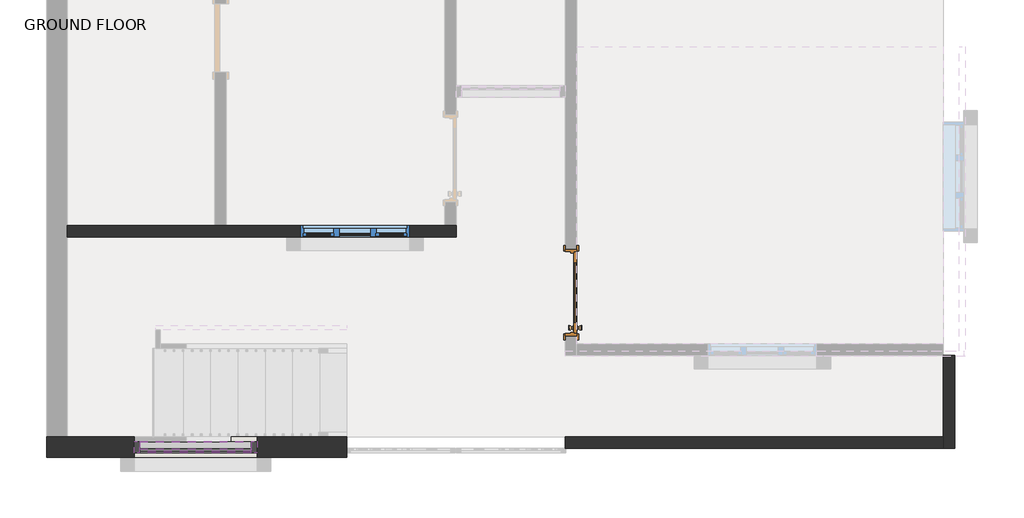
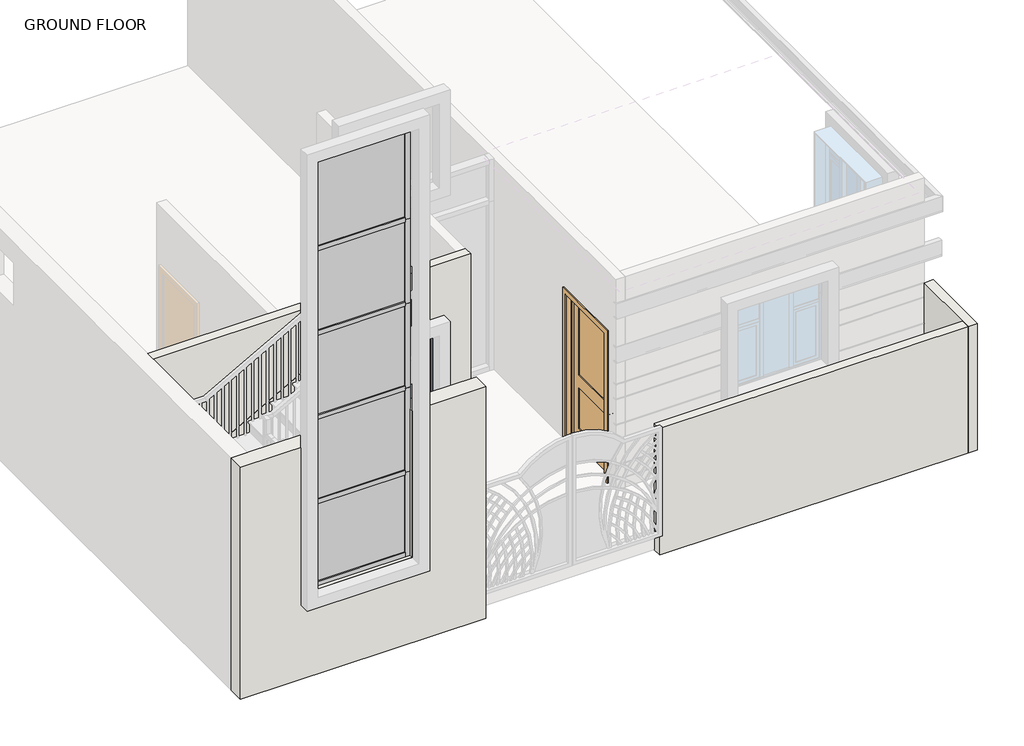
# One storey, part 1 of 7: 16 members, 5 plates, 4 walls, 1 door, 1 window.
"""IFC4 building model written with IfcOpenShell, lengths in millimetres."""

from ifc_helpers import new_model, si_unit, origin, origin_with_axes, place, context, project, spatial, polyline, outline, extrude, faceted_brep, transform, mapped, element, save
from components import door_2e56f206, member_71eb4692, member_a1da5be3, member_0052055d, member_75074519, system_panel_glazed_a6784857, system_panel_glazed_7816ce66, system_panel_glazed_652821f2, window_casement_triple_side_transom_window_4_x_4_9406f89d

model = new_model("IFC4")

# Units and contexts
model_context = context("Model", 3, world=origin())
ifc_project = project(units=[si_unit("LENGTHUNIT", "METRE", prefix="MILLI")], contexts=[model_context])

# Site, building, storey
site = spatial("IfcSite", under=ifc_project)
building = spatial("IfcBuilding", under=site)
storey = spatial("IfcBuildingStorey", under=building, Name="GROUND FLOOR", Elevation=304.8)

# Door
placement = place(None, origin())
door_shape = door_2e56f206(model_context)
element("IfcDoor", 1, ObjectType="Door-Interior-Single-2_Panel-Wood : 36\" x 84\"", at=placement, inside=storey, context=model_context, shape_type="MappedRepresentation", body=[
    mapped(door_shape, transform((-9131.4273867, -1143.8499863, 304.8), x_axis=(0.0, 1.0, 0.0), y_axis=(-1.0, 0.0, 0.0), z_axis=(0.0, 0.0, 1.0))),
])

# Members
member_shape = member_71eb4692(model_context)
element("IfcMember", 2, ObjectType="Rectangular Mullion : 2.5\" x 5\" rectangular", at=placement, inside=storey, context=model_context, shape_type="MappedRepresentation", body=[
    mapped(member_shape, transform((-13947.9023867, -2871.0499863, 7520.3640825), x_axis=(0.0, 0.0, 1.0), y_axis=(0.0, 1.0, 0.0), z_axis=(-1.0, 0.0, 0.0))),
])
element("IfcMember", 3, ObjectType="Rectangular Mullion : 2.5\" x 5\" rectangular", at=placement, inside=storey, context=model_context, shape_type="MappedRepresentation", body=[
    mapped(member_shape, transform((-12703.3023867, -2871.0499863, 1230.3220303), x_axis=(0.0, 0.0, -1.0), y_axis=(0.0, 1.0, 0.0), z_axis=(1.0, 0.0, 0.0))),
])
member_2_shape = member_a1da5be3(model_context)
element("IfcMember", 4, ObjectType="Rectangular Mullion : 2.5\" x 5\" rectangular", at=placement, inside=storey, context=model_context, shape_type="MappedRepresentation", body=[
    mapped(member_2_shape, transform((-13947.9023867, -2871.0499863, 3668.7220303), x_axis=(0.0, 0.0, 1.0), y_axis=(0.0, 1.0, 0.0), z_axis=(-1.0, 0.0, 0.0))),
])
element("IfcMember", 5, ObjectType="Rectangular Mullion : 2.5\" x 5\" rectangular", at=placement, inside=storey, context=model_context, shape_type="MappedRepresentation", body=[
    mapped(member_2_shape, transform((-13947.9023867, -2871.0499863, 6107.1220303), x_axis=(0.0, 0.0, 1.0), y_axis=(0.0, 1.0, 0.0), z_axis=(-1.0, 0.0, 0.0))),
])
element("IfcMember", 6, ObjectType="Rectangular Mullion : 2.5\" x 5\" rectangular", at=placement, inside=storey, context=model_context, shape_type="MappedRepresentation", body=[
    mapped(member_2_shape, transform((-13947.9023867, -2871.0499863, 4887.9220303), x_axis=(0.0, 0.0, 1.0), y_axis=(0.0, 1.0, 0.0), z_axis=(-1.0, 0.0, 0.0))),
])
element("IfcMember", 7, ObjectType="Rectangular Mullion : 2.5\" x 5\" rectangular", at=placement, inside=storey, context=model_context, shape_type="MappedRepresentation", body=[
    mapped(member_2_shape, transform((-13947.9023867, -2871.0499863, 2449.5220303), x_axis=(0.0, 0.0, 1.0), y_axis=(0.0, 1.0, 0.0), z_axis=(-1.0, 0.0, 0.0))),
])
member_3_shape = member_0052055d(model_context)
element("IfcMember", 8, ObjectType="Rectangular Mullion : 2.5\" x 5\" rectangular", at=placement, inside=storey, context=model_context, shape_type="MappedRepresentation", body=[
    mapped(member_3_shape, transform((-12639.8023867, -2871.0499863, 7520.3640825), x_axis=(1.0, 0.0, 0.0), y_axis=(0.0, 1.0, 0.0), z_axis=(0.0, 0.0, 1.0))),
])
element("IfcMember", 9, ObjectType="Rectangular Mullion : 2.5\" x 5\" rectangular", at=placement, inside=storey, context=model_context, shape_type="MappedRepresentation", body=[
    mapped(member_3_shape, transform((-14011.4023867, -2871.0499863, 6107.1220303), x_axis=(-1.0, 0.0, 0.0), y_axis=(0.0, 1.0, 0.0), z_axis=(0.0, 0.0, -1.0))),
])
member_4_shape = member_75074519(model_context)
element("IfcMember", 10, ObjectType="Rectangular Mullion : 2.5\" x 5\" rectangular", at=placement, inside=storey, context=model_context, shape_type="MappedRepresentation", body=[
    mapped(member_4_shape, transform((-14011.4023867, -2871.0499863, 3668.7220303), x_axis=(-1.0, 0.0, 0.0), y_axis=(0.0, 1.0, 0.0), z_axis=(0.0, 0.0, -1.0))),
])
element("IfcMember", 11, ObjectType="Rectangular Mullion : 2.5\" x 5\" rectangular", at=placement, inside=storey, context=model_context, shape_type="MappedRepresentation", body=[
    mapped(member_4_shape, transform((-14011.4023867, -2871.0499863, 4887.9220303), x_axis=(-1.0, 0.0, 0.0), y_axis=(0.0, 1.0, 0.0), z_axis=(0.0, 0.0, -1.0))),
])
element("IfcMember", 12, ObjectType="Rectangular Mullion : 2.5\" x 5\" rectangular", at=placement, inside=storey, context=model_context, shape_type="MappedRepresentation", body=[
    mapped(member_4_shape, transform((-14011.4023867, -2871.0499863, 2449.5220303), x_axis=(-1.0, 0.0, 0.0), y_axis=(0.0, 1.0, 0.0), z_axis=(0.0, 0.0, -1.0))),
])
element("IfcMember", 13, ObjectType="Rectangular Mullion : 2.5\" x 5\" rectangular", at=placement, inside=storey, context=model_context, shape_type="MappedRepresentation", body=[
    mapped(member_4_shape, transform((-12639.8023867, -2871.0499863, 3668.7220303), x_axis=(1.0, 0.0, 0.0), y_axis=(0.0, 1.0, 0.0), z_axis=(0.0, 0.0, 1.0))),
])
element("IfcMember", 14, ObjectType="Rectangular Mullion : 2.5\" x 5\" rectangular", at=placement, inside=storey, context=model_context, shape_type="MappedRepresentation", body=[
    mapped(member_4_shape, transform((-12639.8023867, -2871.0499863, 6107.1220303), x_axis=(1.0, 0.0, 0.0), y_axis=(0.0, 1.0, 0.0), z_axis=(0.0, 0.0, 1.0))),
])
element("IfcMember", 15, ObjectType="Rectangular Mullion : 2.5\" x 5\" rectangular", at=placement, inside=storey, context=model_context, shape_type="MappedRepresentation", body=[
    mapped(member_4_shape, transform((-12639.8023867, -2871.0499863, 4887.9220303), x_axis=(1.0, 0.0, 0.0), y_axis=(0.0, 1.0, 0.0), z_axis=(0.0, 0.0, 1.0))),
])
element("IfcMember", 16, ObjectType="Rectangular Mullion : 2.5\" x 5\" rectangular", at=placement, inside=storey, context=model_context, shape_type="MappedRepresentation", body=[
    mapped(member_4_shape, transform((-14011.4023867, -2871.0499863, 1230.3220303), x_axis=(-1.0, 0.0, 0.0), y_axis=(0.0, 1.0, 0.0), z_axis=(0.0, 0.0, -1.0))),
])
element("IfcMember", 17, ObjectType="Rectangular Mullion : 2.5\" x 5\" rectangular", at=placement, inside=storey, context=model_context, shape_type="MappedRepresentation", body=[
    mapped(member_4_shape, transform((-12639.8023867, -2871.0499863, 2449.5220303), x_axis=(1.0, 0.0, 0.0), y_axis=(0.0, 1.0, 0.0), z_axis=(0.0, 0.0, 1.0))),
])

# Plates
system_panel_glazed_shape = system_panel_glazed_a6784857(model_context)
element("IfcPlate", 18, ObjectType="System Panel : Glazed", at=placement, inside=storey, context=model_context, shape_type="MappedRepresentation", body=[
    mapped(system_panel_glazed_shape, transform((-13325.6023867, -2871.0499863, 6138.8720303), x_axis=(-1.0, 0.0, 0.0), y_axis=(0.0, -1.0, 0.0), z_axis=(0.0, 0.0, 1.0))),
])
system_panel_glazed_2_shape = system_panel_glazed_7816ce66(model_context)
element("IfcPlate", 19, ObjectType="System Panel : Glazed", at=placement, inside=storey, context=model_context, shape_type="MappedRepresentation", body=[
    mapped(system_panel_glazed_2_shape, transform((-13325.6023867, -2871.0499863, 3700.4720303), x_axis=(-1.0, 0.0, 0.0), y_axis=(0.0, -1.0, 0.0), z_axis=(0.0, 0.0, 1.0))),
])
element("IfcPlate", 20, ObjectType="System Panel : Glazed", at=placement, inside=storey, context=model_context, shape_type="MappedRepresentation", body=[
    mapped(system_panel_glazed_2_shape, transform((-13325.6023867, -2871.0499863, 4919.6720303), x_axis=(-1.0, 0.0, 0.0), y_axis=(0.0, -1.0, 0.0), z_axis=(0.0, 0.0, 1.0))),
])
element("IfcPlate", 21, ObjectType="System Panel : Glazed", at=placement, inside=storey, context=model_context, shape_type="MappedRepresentation", body=[
    mapped(system_panel_glazed_2_shape, transform((-13325.6023867, -2871.0499863, 2481.2720303), x_axis=(-1.0, 0.0, 0.0), y_axis=(0.0, -1.0, 0.0), z_axis=(0.0, 0.0, 1.0))),
])
system_panel_glazed_3_shape = system_panel_glazed_652821f2(model_context)
element("IfcPlate", 22, ObjectType="System Panel : Glazed", at=placement, inside=storey, context=model_context, shape_type="MappedRepresentation", body=[
    mapped(system_panel_glazed_3_shape, transform((-13325.6023867, -2871.0499863, 1293.8220303), x_axis=(-1.0, 0.0, 0.0), y_axis=(0.0, -1.0, 0.0), z_axis=(0.0, 0.0, 1.0))),
])

# Walls
element("IfcWall", 23, at=placement, inside=storey, context=model_context, shape_type="Brep", body=[
    faceted_brep([(-11636.5023867, -2756.7499863, 0.0), (-14760.7023867, -2756.7499863, 0.0), (-14989.3023867, -2756.7499863, 0.0), (-14989.3023867, -2756.7499863, 3352.8), (-14760.7023867, -2756.7499863, 3352.8), (-14011.4023867, -2756.7499863, 3352.8), (-14011.4023867, -2756.7499863, 1230.3220303), (-12639.8023867, -2756.7499863, 1230.3220303), (-12639.8023867, -2756.7499863, 3352.8), (-11636.5023867, -2756.7499863, 3352.8), (-14989.3023867, -2985.3499863, 0.0), (-11636.5023867, -2985.3499863, 0.0), (-11636.5023867, -2985.3499863, 3352.8), (-12639.8023867, -2985.3499863, 3352.8), (-12639.8023867, -2985.3499863, 1230.3220303), (-14011.4023867, -2985.3499863, 1230.3220303), (-14011.4023867, -2985.3499863, 3352.8), (-14989.3023867, -2985.3499863, 3352.8)], [[[0, 1, 2, 3, 4, 5, 6, 7, 8, 9]], [[10, 11, 12, 13, 14, 15, 16, 17]], [[2, 1, 0, 11, 10]], [[12, 9, 8, 13]], [[3, 17, 16, 5, 4]], [[0, 9, 12, 11]], [[3, 2, 10, 17]], [[7, 14, 13, 8]], [[15, 6, 5, 16]], [[14, 7, 6, 15]]]),
])
element("IfcWall", 24, ObjectType="INNER WALL 5\"", at=placement, inside=storey, context=model_context, shape_type="Brep", body=[
    faceted_brep([(-14760.7023867, -521.5499863, 304.8), (-10417.3023867, -521.5499863, 304.8), (-10417.3023867, -521.5499863, 3352.8), (-14760.7023867, -521.5499863, 3352.8), (-12157.2023867, -521.5499863, 2438.4), (-10938.0023867, -521.5499863, 2438.4), (-10938.0023867, -521.5499863, 1219.2), (-12157.2023867, -521.5499863, 1219.2), (-14760.7023867, -394.5499863, 304.8), (-14760.7023867, -394.5499863, 3352.8), (-13109.7023867, -394.5499863, 3352.8), (-12982.7023867, -394.5499863, 3352.8), (-10544.3023867, -394.5499863, 3352.8), (-10417.3023867, -394.5499863, 3352.8), (-10417.3023867, -394.5499863, 304.8), (-10544.3023867, -394.5499863, 304.8), (-12982.7023867, -394.5499863, 304.8), (-13109.7023867, -394.5499863, 304.8), (-12157.2023867, -394.5499863, 2438.4), (-12157.2023867, -394.5499863, 1219.2), (-10938.0023867, -394.5499863, 1219.2), (-10938.0023867, -394.5499863, 2438.4)], [[[0, 1, 2, 3], [4, 5, 6, 7]], [[8, 9, 10, 11, 12, 13, 14, 15, 16, 17], [18, 19, 20, 21]], [[1, 0, 8, 17, 16, 15, 14]], [[3, 2, 13, 12, 11, 10, 9]], [[0, 3, 9, 8]], [[2, 1, 14, 13]], [[19, 18, 4, 7]], [[20, 19, 7, 6]], [[21, 20, 6, 5]], [[18, 21, 5, 4]]]),
])
element("IfcWall", 25, ObjectType="INNER WALL 5\"", at=placement, inside=storey, context=model_context, shape_type="Brep", body=[
    faceted_brep([(-4981.7023867, -1842.3499863, 0.0), (-4981.7023867, -2756.7499863, 0.0), (-4981.7023867, -2883.7499863, 0.0), (-4981.7023867, -2883.7499863, 1828.8), (-4981.7023867, -2756.7499863, 1828.8), (-4981.7023867, -1842.3499863, 1828.8), (-4854.7023867, -1842.3499863, 0.0), (-4854.7023867, -1842.3499863, 1828.8), (-4854.7023867, -2883.7499863, 1828.8), (-4854.7023867, -2883.7499863, 0.0)], [[[0, 1, 2, 3, 4, 5]], [[6, 7, 8, 9]], [[2, 1, 0, 6, 9]], [[5, 4, 3, 8, 7]], [[0, 5, 7, 6]], [[3, 2, 9, 8]]]),
])
element("IfcWall", 26, ObjectType="INNER WALL 5\"", at=placement, inside=storey, context=model_context, shape_type="SweptSolid", body=[
    extrude(outline(polyline([(-9198.1023867, -2756.7499863), (-4981.7023867, -2756.7499863), (-4981.7023867, -2883.7499863), (-9198.1023867, -2883.7499863), (-9198.1023867, -2756.7499863)])), origin_with_axes(), (0.0, 0.0, 1.0), 1828.8),
])

# Window
window_casement_triple_side_transom_window_4_x_4_shape = window_casement_triple_side_transom_window_4_x_4_9406f89d(model_context)
element("IfcWindow", 27, ObjectType="Window-Casement-Triple-Side-Transom : window 4' x 4'", at=placement, inside=storey, context=model_context, shape_type="MappedRepresentation", body=[
    mapped(window_casement_triple_side_transom_window_4_x_4_shape, transform((-11547.6023867, -458.0499863, 304.8), x_axis=(-1.0, 0.0, 0.0), y_axis=(0.0, -1.0, 0.0), z_axis=(0.0, 0.0, 1.0))),
])

save(model, "model.ifc")

# Revit data of these elements
# Type "Door-Interior-Single-2_Panel-Wood : 36\" x 84\""
#   Type Mark = "8"
#   Assembly Code = "C1020300"
#   Analytic Construction = "Wooden"
#   Top Rail = 0' - 4 11/16"
#   Thickness = 0' - 1 3/8"
#   Thermal Resistance (R) = 2.5876 (h·ft²·°F)/BTU
#   Swing Angle [instance default] = 90.00°
#   Stiles = 0' - 4 3/4"
#   Rough Width = 3' - 2"
#   Rough Height = 7' - 1"
#   Lock Rail = 0' - 7 1/2"
#   Height = 7' - 0"
#   Width = 3' - 0"
#   Heat Transfer Coefficient (U) = 0.3865 BTU/(h·ft²·°F)
#   Bottom Rail = 0' - 9 1/8"
#   Trim Material = Cherry
#   Panel Material = Cherry
#   Frame Material = Cherry
#   Door Handle Material = Aluminum
#   Visual Light Transmittance = 0
#   Solar Heat Gain Coefficient = 0
#   Wall Closure = (empty or 0)
#   Function = (empty or 0)
# Type "Rectangular Mullion : 2.5\" x 5\" rectangular"
#   built-in parameter 1007304 = 0.416667 (stored number, unit not read)
#   built-in parameter 1007301 = 0.104167 (stored number, unit not read)
#   built-in parameter 1007300 = 0.104167 (stored number, unit not read)
# Type "System Panel : Glazed"
#   Construction Type Id = "GSP4R"
#   Analytic Construction = "1/8 in Pilkington single glazing"
#   Visual Light Transmittance = 0.9
#   Solar Heat Gain Coefficient = 0.86
#   Heat Transfer Coefficient (U) = 1.18115 BTU/(h·ft²·°F)
#   Define Thermal Properties by = 1
# Type
#   Assembly Code = "B2010"
#   Layers, outside or top first: 0' - 9" "OUTER WALL" (function 1)
# Type "INNER WALL 5\""
#   Assembly Code = "B2010"
#   Layers, outside or top first: 0' - 5" "OUTER WALL" (function 1)
# Type "Window-Casement-Triple-Side-Transom : window 4' x 4'"
#   Type Mark = "22"
#   Fire Rating = "0.5h"
#   Assembly Code = "B2020100"
#   Analytic Construction = "Double glazing - domestic"
#   Window Width = 1' - 4"
#   Window Inset [instance default] = 0' - 0 5/8"
#   Wall Thickness [instance default] = 0' - 6"
#   Visual Light Transmittance = 0.81
#   Transom Height Ratio = 0.3
#   Thermal Resistance (R) = 1.8146 (h·ft²·°F)/BTU
#   Solar Heat Gain Coefficient = 0.76
#   Rough Width = 4' - 0 1/2"
#   Rough Height = 4' - 0 1/2"
#   Open Window Height = 2' - 9.6"
#   Heat Transfer Coefficient (U) = 0.5511 BTU/(h·ft²·°F)
#   Height = 4' - 0"
#   Transom Height = 1' - 2.4"
#   Frame Gap 3 [instance default] = 0' - 1 83/128"
#   Frame Gap 2 [instance default] = 0' - 0 5/8"
#   Frame Gap 1 = 0' - 1 51/128"
#   Default Sill Height = 3' - 0"
#   Width = 4' - 0"
#   Frame Material = Metal - Aluminum
#   Glass Panel Material = Glass
#   Wall Closure = (empty or 0)
# Element 1 (IfcDoor, "Door-Interior-Single-2_Panel-Wood : 36\" x 84\"")
#   Swing Angle = 90.00°
#   Phase Created = New Construction
#   Materials on its faces: "Cherry", "Aluminum"
# Elements 2, 3, 4, 5, 6, 7, 8, 9, 10, 11, 12, 13, 14, 15, 16, 17 (IfcMember, "Rectangular Mullion : 2.5\" x 5\" rectangular")
#   Phase Created = New Construction
#   Materials on its faces: "Aluminum"
# Elements 18, 19, 20, 21, 22 (IfcPlate, "System Panel : Glazed")
#   Phase Created = New Construction
#   Materials on its faces: "Glass"
# Element 23 (IfcWall)
#   built-in parameter 1001111 = -1' - 0"
#   Top Offset = 0' - 0"
#   Base Offset = -1' - 0"
#   wall height = 11' - 0"
#   Phase Created = New Construction
#   Base Constraint = GROUND FLOOR
#   Top Constraint = FIRST FLOOR
#   Materials on its faces: "OUTER WALL"
# Element 24 (IfcWall, "INNER WALL 5\"")
#   Top Offset = 0' - 0"
#   Base Offset = 0' - 0"
#   wall height = 10' - 0"
#   Phase Created = New Construction
#   Base Constraint = GROUND FLOOR
#   Top Constraint = FIRST FLOOR
#   Materials on its faces: "OUTER WALL"
# Elements 25, 26 (IfcWall, "INNER WALL 5\"")
#   built-in parameter 1001111 = -1' - 0"
#   Top Offset = 0' - 0"
#   Base Offset = -1' - 0"
#   Unconnected Height = 6' - 0"
#   wall height = 6' - 0"
#   Phase Created = New Construction
#   Base Constraint = GROUND FLOOR
#   Materials on its faces: "OUTER WALL"
# Element 27 (IfcWindow, "Window-Casement-Triple-Side-Transom : window 4' x 4'")
#   Mark = "9"
#   Window Inset = 0' - 0 5/8"
#   Frame Gap 3 = 0' - 1 83/128"
#   Frame Gap 2 = 0' - 0 5/8"
#   Phase Created = New Construction
#   Materials on its faces: "Metal - Aluminum", "Glass"
# Materials
#   "Cherry": class "Wood", colour RGB 226 177 128, transparency 0, Description = "Prunus Serotina", Cost = 0
#   "Aluminum": class "Metal", colour RGB 247 247 247, transparency 0, Description = "Aluminum 6061", Cost = 0
#   "OUTER WALL": class "Generic", colour RGB 245 245 240, transparency 0, Cost = 0
#   "Metal - Aluminum": class "Metal", colour RGB 247 247 247, transparency 0
#   "Glass": class "Glass", colour RGB 0 128 192, transparency 0.75, Description = "Soda Lime Glass", Cost = 0
